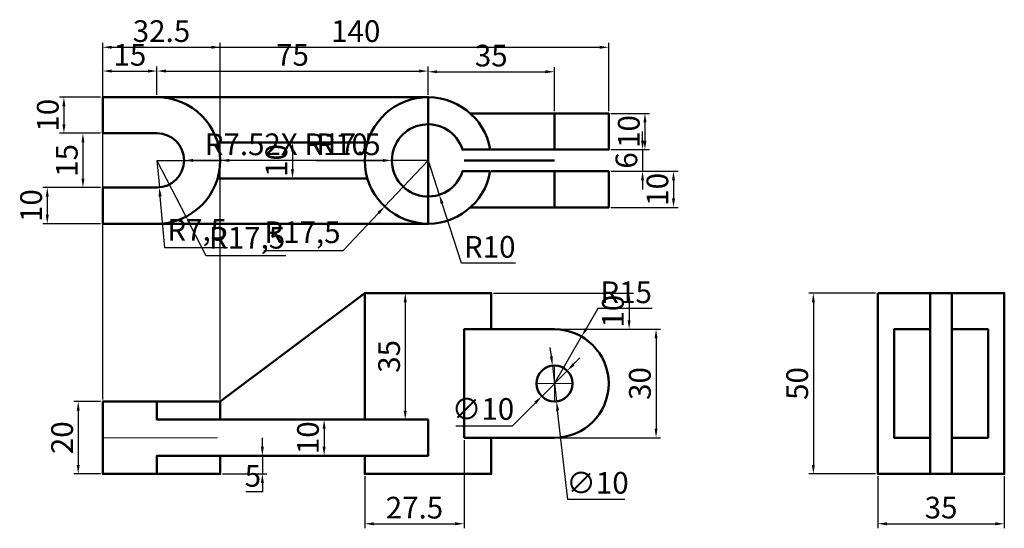
# Model space of a CAD drawing. Units: millimetres. Extents: x 147 to 419, y 95 to 236.
import ezdxf

# ---------------------------------------------------------------- set-up
doc = ezdxf.new("R2010")
doc.units = ezdxf.units.MM
doc.linetypes.add('CENTER', pattern=[50.8, 31.75, -6.35, 6.35, -6.35])
for name, color, linetype, lineweight in [('M-CNTR', 1, 'CENTER', 18), ('M-DIMS', 2, 'Continuous', 25), ('M-OUTL', 7, 'Continuous', 50)]:
    doc.layers.add(name, color=color, linetype=linetype, lineweight=lineweight)
doc.styles.get("Standard").update_dxf_attribs({"font": 'arial.ttf'})
doc.dimstyles.new('ISO-25', dxfattribs={"dimtxt": 6, "dimasz": 2.5, "dimexe": 1.25, "dimexo": 0.625, "dimtad": 1, "dimtoh": 1, "dimdec": 1, "dimtxsty": 'Standard', "dimcen": 2.5, "dimadec": 0, "dimazin": 0, "dimtfac": 1, "dimtdec": 1, "dimtmove": 0, "dimatfit": 3, "dimfxl": 1, "dimarcsym": 0})

# ---------------------------------------------------------------- blocks, each defined once
blk = doc.blocks.new('*D1')
at = {"layer": 'Defpoints', "color": 0, "transparency": 16777216}
for p in [(384.43, 159.98), (366.59, 109.98), (384.43, 109.98)]:
    blk.add_point(p, dxfattribs=at)
at = {"layer": 'M-DIMS', "color": 0, "lineweight": -2, "transparency": 16777216}
for p, q in [((383.8, 159.98), (365.34, 159.98)), ((366.59, 157.48), (366.59, 112.48)), ((383.8, 109.98), (365.34, 109.98))]:
    blk.add_line(p, q, dxfattribs=at)
at = {"layer": 'M-DIMS', "color": 0, "transparency": 16777216}
for points in [[(366.17, 157.48), (367.01, 157.48), (366.59, 159.98)], [(366.17, 112.48), (367.01, 112.48), (366.59, 109.98)]]:
    blk.add_solid(points, dxfattribs=at)
at = {"layer": 'M-DIMS', "color": 0, "transparency": 16777216, "insert": (362.9, 134.98), "char_height": 6, "attachment_point": 5, "rotation": 90}
blk.add_mtext('50', dxfattribs=at)
blk = doc.blocks.new('*D2')
at = {"layer": 'Defpoints', "color": 0, "transparency": 16777216}
for p in [(294.96, 149.98), (294.96, 119.98), (323.06, 119.98)]:
    blk.add_point(p, dxfattribs=at)
at = {"layer": 'M-DIMS', "color": 0, "lineweight": -2, "transparency": 16777216}
for p, q in [((295.58, 149.98), (324.31, 149.98)), ((323.06, 147.48), (323.06, 122.48)), ((295.58, 119.98), (324.31, 119.98))]:
    blk.add_line(p, q, dxfattribs=at)
at = {"layer": 'M-DIMS', "color": 0, "transparency": 16777216}
for points in [[(322.64, 147.48), (323.48, 147.48), (323.06, 149.98)], [(322.64, 122.48), (323.48, 122.48), (323.06, 119.98)]]:
    blk.add_solid(points, dxfattribs=at)
at = {"layer": 'M-DIMS', "color": 0, "transparency": 16777216, "insert": (319.37, 134.98), "char_height": 6, "attachment_point": 5, "rotation": 90}
blk.add_mtext('30', dxfattribs=at)
blk = doc.blocks.new('*D3')
at = {"layer": 'Defpoints', "color": 0, "transparency": 16777216}
for p in [(277.46, 159.98), (277.46, 149.98), (315.6, 149.98)]:
    blk.add_point(p, dxfattribs=at)
at = {"layer": 'M-DIMS', "color": 0, "lineweight": -2, "transparency": 16777216}
for p, q in [((278.08, 159.98), (316.85, 159.98)), ((315.6, 157.48), (315.6, 152.48)), ((278.08, 149.98), (316.85, 149.98))]:
    blk.add_line(p, q, dxfattribs=at)
at = {"layer": 'M-DIMS', "color": 0, "transparency": 16777216}
for points in [[(315.18, 157.48), (316.01, 157.48), (315.6, 159.98)], [(315.18, 152.48), (316.01, 152.48), (315.6, 149.98)]]:
    blk.add_solid(points, dxfattribs=at)
at = {"layer": 'M-DIMS', "color": 0, "transparency": 16777216, "insert": (311.91, 154.98), "char_height": 6, "attachment_point": 5, "rotation": 90}
blk.add_mtext('10', dxfattribs=at)
blk = doc.blocks.new('*D4')
at = {"layer": 'Defpoints', "color": 0, "transparency": 16777216}
for p in [(294.38, 139.94), (295.53, 130.01)]:
    blk.add_point(p, dxfattribs=at)
at = {"layer": 'M-DIMS', "color": 0, "lineweight": -2, "transparency": 16777216}
for p, q in [((294.09, 142.43), (293.8, 144.91)), ((294.38, 139.94), (295.53, 130.01)), ((298.68, 102.87), (295.82, 127.53)), ((314.41, 102.87), (298.68, 102.87))]:
    blk.add_line(p, q, dxfattribs=at)
at = {"layer": 'M-DIMS', "color": 0, "transparency": 16777216}
for points in [[(294.51, 142.47), (293.68, 142.38), (294.38, 139.94)], [(296.24, 127.57), (295.41, 127.48), (295.53, 130.01)]]:
    blk.add_solid(points, dxfattribs=at)
at = {"layer": 'M-DIMS', "color": 0, "transparency": 16777216, "insert": (306.86, 106.73), "char_height": 6, "attachment_point": 5}
blk.add_mtext('∅10', dxfattribs=at)
blk = doc.blocks.new('*D5')
at = {"layer": 'Defpoints', "color": 0, "transparency": 16777216}
for p in [(259.96, 159.98), (253.66, 124.98), (259.96, 124.98)]:
    blk.add_point(p, dxfattribs=at)
at = {"layer": 'M-DIMS', "color": 0, "lineweight": -2, "transparency": 16777216}
for p, q in [((259.33, 159.98), (252.41, 159.98)), ((253.66, 157.48), (253.66, 127.48)), ((259.33, 124.98), (252.41, 124.98))]:
    blk.add_line(p, q, dxfattribs=at)
at = {"layer": 'M-DIMS', "color": 0, "transparency": 16777216}
for points in [[(253.24, 157.48), (254.07, 157.48), (253.66, 159.98)], [(253.24, 127.48), (254.07, 127.48), (253.66, 124.98)]]:
    blk.add_solid(points, dxfattribs=at)
at = {"layer": 'M-DIMS', "color": 0, "transparency": 16777216, "insert": (249.97, 142.48), "char_height": 6, "attachment_point": 5, "rotation": 90}
blk.add_mtext('35', dxfattribs=at)
blk = doc.blocks.new('*D6')
at = {"layer": 'Defpoints', "color": 0, "transparency": 16777216}
for p in [(231.21, 124.98), (231.21, 114.98), (231.21, 114.98)]:
    blk.add_point(p, dxfattribs=at)
at = {"layer": 'M-DIMS', "color": 0, "lineweight": -2, "transparency": 16777216}
for p, q in [((231.83, 124.98), (232.46, 124.98)), ((231.21, 122.48), (231.21, 117.48)), ((231.83, 114.98), (232.46, 114.98))]:
    blk.add_line(p, q, dxfattribs=at)
at = {"layer": 'M-DIMS', "color": 0, "transparency": 16777216}
for points in [[(230.79, 122.48), (231.62, 122.48), (231.21, 124.98)], [(230.79, 117.48), (231.62, 117.48), (231.21, 114.98)]]:
    blk.add_solid(points, dxfattribs=at)
at = {"layer": 'M-DIMS', "color": 0, "transparency": 16777216, "insert": (227.52, 119.98), "char_height": 6, "attachment_point": 5, "rotation": 90}
blk.add_mtext('10', dxfattribs=at)
blk = doc.blocks.new('*D7')
at = {"layer": 'Defpoints', "color": 0, "transparency": 16777216}
for p in [(169.96, 129.98), (163.17, 109.98), (169.96, 109.98)]:
    blk.add_point(p, dxfattribs=at)
at = {"layer": 'M-DIMS', "color": 0, "lineweight": -2, "transparency": 16777216}
for p, q in [((169.33, 129.98), (161.92, 129.98)), ((163.17, 127.48), (163.17, 112.48)), ((169.33, 109.98), (161.92, 109.98))]:
    blk.add_line(p, q, dxfattribs=at)
at = {"layer": 'M-DIMS', "color": 0, "transparency": 16777216}
for points in [[(162.75, 127.48), (163.58, 127.48), (163.17, 129.98)], [(162.75, 112.48), (163.58, 112.48), (163.17, 109.98)]]:
    blk.add_solid(points, dxfattribs=at)
at = {"layer": 'M-DIMS', "color": 0, "transparency": 16777216, "insert": (159.48, 119.98), "char_height": 6, "attachment_point": 5, "rotation": 90}
blk.add_mtext('20', dxfattribs=at)
blk = doc.blocks.new('*D8')
at = {"layer": 'Defpoints', "color": 0, "transparency": 16777216}
for p in [(202.46, 114.98), (202.46, 109.98), (214.12, 109.98)]:
    blk.add_point(p, dxfattribs=at)
at = {"layer": 'M-DIMS', "color": 0, "lineweight": -2, "transparency": 16777216}
for p, q in [((214.12, 117.48), (214.12, 119.98)), ((203.08, 114.98), (215.37, 114.98)), ((214.12, 114.98), (214.12, 109.98)), ((203.08, 109.98), (215.37, 109.98)), ((214.12, 107.48), (214.12, 104.98)), ((214.12, 104.98), (209.52, 104.98))]:
    blk.add_line(p, q, dxfattribs=at)
at = {"layer": 'M-DIMS', "color": 0, "transparency": 16777216}
for points in [[(213.71, 117.48), (214.54, 117.48), (214.12, 114.98)], [(213.71, 107.48), (214.54, 107.48), (214.12, 109.98)]]:
    blk.add_solid(points, dxfattribs=at)
at = {"layer": 'M-DIMS', "color": 0, "transparency": 16777216, "insert": (211.51, 108.65), "char_height": 6, "attachment_point": 5}
blk.add_mtext('5', dxfattribs=at)
blk = doc.blocks.new('*D9')
at = {"layer": 'Defpoints', "color": 0, "transparency": 16777216}
for p in [(169.96, 214.19), (159.21, 204.19), (169.96, 204.19)]:
    blk.add_point(p, dxfattribs=at)
at = {"layer": 'M-DIMS', "color": 0, "lineweight": -2, "transparency": 16777216}
for p, q in [((169.33, 214.19), (157.96, 214.19)), ((159.21, 211.69), (159.21, 206.69)), ((169.33, 204.19), (157.96, 204.19))]:
    blk.add_line(p, q, dxfattribs=at)
at = {"layer": 'M-DIMS', "color": 0, "transparency": 16777216}
for points in [[(158.8, 211.69), (159.63, 211.69), (159.21, 214.19)], [(158.8, 206.69), (159.63, 206.69), (159.21, 204.19)]]:
    blk.add_solid(points, dxfattribs=at)
at = {"layer": 'M-DIMS', "color": 0, "transparency": 16777216, "insert": (155.52, 209.19), "char_height": 6, "attachment_point": 5, "rotation": 90}
blk.add_mtext('10', dxfattribs=at)
blk = doc.blocks.new('*D10')
at = {"layer": 'Defpoints', "color": 0, "transparency": 16777216}
for p in [(169.96, 204.19), (164.48, 189.19), (169.96, 189.19)]:
    blk.add_point(p, dxfattribs=at)
at = {"layer": 'M-DIMS', "color": 0, "lineweight": -2, "transparency": 16777216}
for p, q in [((169.33, 204.19), (163.23, 204.19)), ((164.48, 201.69), (164.48, 191.69)), ((169.33, 189.19), (163.23, 189.19))]:
    blk.add_line(p, q, dxfattribs=at)
at = {"layer": 'M-DIMS', "color": 0, "transparency": 16777216}
for points in [[(164.07, 201.69), (164.9, 201.69), (164.48, 204.19)], [(164.07, 191.69), (164.9, 191.69), (164.48, 189.19)]]:
    blk.add_solid(points, dxfattribs=at)
at = {"layer": 'M-DIMS', "color": 0, "transparency": 16777216, "insert": (160.79, 196.69), "char_height": 6, "attachment_point": 5, "rotation": 90}
blk.add_mtext('15', dxfattribs=at)
blk = doc.blocks.new('*D11')
at = {"layer": 'Defpoints', "color": 0, "transparency": 16777216}
for p in [(169.96, 189.19), (154.6, 179.19), (169.96, 179.19)]:
    blk.add_point(p, dxfattribs=at)
at = {"layer": 'M-DIMS', "color": 0, "lineweight": -2, "transparency": 16777216}
for p, q in [((169.33, 189.19), (153.35, 189.19)), ((154.6, 186.69), (154.6, 181.69)), ((169.33, 179.19), (153.35, 179.19))]:
    blk.add_line(p, q, dxfattribs=at)
at = {"layer": 'M-DIMS', "color": 0, "transparency": 16777216}
for points in [[(154.18, 186.69), (155.02, 186.69), (154.6, 189.19)], [(154.18, 181.69), (155.02, 181.69), (154.6, 179.19)]]:
    blk.add_solid(points, dxfattribs=at)
at = {"layer": 'M-DIMS', "color": 0, "transparency": 16777216, "insert": (150.91, 184.19), "char_height": 6, "attachment_point": 5, "rotation": 90}
blk.add_mtext('10', dxfattribs=at)
blk = doc.blocks.new('*D12')
at = {"layer": 'Defpoints', "color": 0, "transparency": 16777216}
for p in [(184.96, 221.42), (169.96, 214.19), (184.96, 214.19)]:
    blk.add_point(p, dxfattribs=at)
at = {"layer": 'M-DIMS', "color": 0, "lineweight": -2, "transparency": 16777216}
for p, q in [((169.96, 214.82), (169.96, 222.67)), ((172.46, 221.42), (182.46, 221.42)), ((184.96, 214.82), (184.96, 222.67))]:
    blk.add_line(p, q, dxfattribs=at)
at = {"layer": 'M-DIMS', "color": 0, "transparency": 16777216}
for points in [[(172.46, 221.84), (172.46, 221), (169.96, 221.42)], [(182.46, 221.84), (182.46, 221), (184.96, 221.42)]]:
    blk.add_solid(points, dxfattribs=at)
at = {"layer": 'M-DIMS', "color": 0, "transparency": 16777216, "insert": (177.46, 225.11), "char_height": 6, "attachment_point": 5}
blk.add_mtext('15', dxfattribs=at)
blk = doc.blocks.new('*D13')
at = {"layer": 'Defpoints', "color": 0, "transparency": 16777216}
for p in [(259.96, 221.42), (184.96, 218.74), (259.96, 214.19)]:
    blk.add_point(p, dxfattribs=at)
at = {"layer": 'M-DIMS', "color": 0, "lineweight": -2, "transparency": 16777216}
for p, q in [((184.96, 219.37), (184.96, 222.67)), ((187.46, 221.42), (257.46, 221.42)), ((259.96, 214.82), (259.96, 222.67))]:
    blk.add_line(p, q, dxfattribs=at)
at = {"layer": 'M-DIMS', "color": 0, "transparency": 16777216}
for points in [[(187.46, 221.84), (187.46, 221), (184.96, 221.42)], [(257.46, 221.84), (257.46, 221), (259.96, 221.42)]]:
    blk.add_solid(points, dxfattribs=at)
at = {"layer": 'M-DIMS', "color": 0, "transparency": 16777216, "insert": (222.46, 225.1), "char_height": 6, "attachment_point": 5}
blk.add_mtext('75', dxfattribs=at)
blk = doc.blocks.new('*D14')
at = {"layer": 'Defpoints', "color": 0, "transparency": 16777216}
for p in [(222.46, 201.69), (222.46, 191.69), (222.46, 191.69)]:
    blk.add_point(p, dxfattribs=at)
at = {"layer": 'M-DIMS', "color": 0, "lineweight": -2, "transparency": 16777216}
for p, q in [((223.08, 201.69), (223.71, 201.69)), ((222.46, 199.19), (222.46, 194.19)), ((223.08, 191.69), (223.71, 191.69))]:
    blk.add_line(p, q, dxfattribs=at)
at = {"layer": 'M-DIMS', "color": 0, "transparency": 16777216}
for points in [[(222.04, 199.19), (222.87, 199.19), (222.46, 201.69)], [(222.04, 194.19), (222.87, 194.19), (222.46, 191.69)]]:
    blk.add_solid(points, dxfattribs=at)
at = {"layer": 'M-DIMS', "color": 0, "transparency": 16777216, "insert": (218.77, 196.69), "char_height": 6, "attachment_point": 5, "rotation": 90}
blk.add_mtext('10', dxfattribs=at)
blk = doc.blocks.new('*D15')
at = {"layer": 'Defpoints', "color": 0, "transparency": 16777216}
for p in [(184.96, 196.69), (192.98, 181.14)]:
    blk.add_point(p, dxfattribs=at)
at = {"layer": 'M-DIMS', "color": 0, "lineweight": -2, "transparency": 16777216}
for p, q in [((184.96, 196.69), (192.98, 181.14)), ((198.58, 170.29), (194.13, 178.92)), ((220.58, 170.29), (198.58, 170.29))]:
    blk.add_line(p, q, dxfattribs=at)
at = {"layer": 'M-DIMS', "color": 0, "transparency": 16777216}
blk.add_solid([(194.5, 179.11), (193.76, 178.73), (192.98, 181.14)], dxfattribs=at)
at = {"layer": 'M-DIMS', "color": 0, "transparency": 16777216, "insert": (209.89, 174.52), "char_height": 6, "attachment_point": 5}
blk.add_mtext('R17,5', dxfattribs=at)
blk = doc.blocks.new('*D16')
at = {"layer": 'Defpoints', "color": 0, "transparency": 16777216}
for p in [(184.96, 196.69), (185.62, 189.22)]:
    blk.add_point(p, dxfattribs=at)
at = {"layer": 'M-DIMS', "color": 0, "lineweight": -2, "transparency": 16777216}
for p, q in [((184.96, 196.69), (185.62, 189.22)), ((187.11, 172.48), (185.84, 186.73)), ((204.44, 172.48), (187.11, 172.48))]:
    blk.add_line(p, q, dxfattribs=at)
at = {"layer": 'M-DIMS', "color": 0, "transparency": 16777216}
blk.add_solid([(186.26, 186.77), (185.43, 186.7), (185.62, 189.22)], dxfattribs=at)
at = {"layer": 'M-DIMS', "color": 0, "transparency": 16777216, "insert": (196.09, 176.7), "char_height": 6, "attachment_point": 5}
blk.add_mtext('R7,5', dxfattribs=at)
blk = doc.blocks.new('*D17')
at = {"layer": 'Defpoints', "color": 0, "transparency": 16777216}
for p in [(259.96, 196.69), (263.07, 187.19)]:
    blk.add_point(p, dxfattribs=at)
at = {"layer": 'M-DIMS', "color": 0, "lineweight": -2, "transparency": 16777216}
for p, q in [((259.96, 196.69), (263.07, 187.19)), ((269.25, 168.31), (263.85, 184.82)), ((284.19, 168.31), (269.25, 168.31))]:
    blk.add_line(p, q, dxfattribs=at)
at = {"layer": 'M-DIMS', "color": 0, "transparency": 16777216}
blk.add_solid([(264.24, 184.95), (263.45, 184.69), (263.07, 187.19)], dxfattribs=at)
at = {"layer": 'M-DIMS', "color": 0, "transparency": 16777216, "insert": (277.03, 172), "char_height": 6, "attachment_point": 5}
blk.add_mtext('R10', dxfattribs=at)
blk = doc.blocks.new('*D18')
at = {"layer": 'Defpoints', "color": 0, "transparency": 16777216}
for p in [(259.96, 196.69), (247.96, 183.96)]:
    blk.add_point(p, dxfattribs=at)
at = {"layer": 'M-DIMS', "color": 0, "lineweight": -2, "transparency": 16777216}
for p, q in [((259.96, 196.69), (247.96, 183.96)), ((236.52, 171.82), (246.24, 182.14)), ((214.53, 171.82), (236.52, 171.82))]:
    blk.add_line(p, q, dxfattribs=at)
at = {"layer": 'M-DIMS', "color": 0, "transparency": 16777216}
blk.add_solid([(245.94, 182.42), (246.55, 181.85), (247.96, 183.96)], dxfattribs=at)
at = {"layer": 'M-DIMS', "color": 0, "transparency": 16777216, "insert": (225.21, 176.05), "char_height": 6, "attachment_point": 5}
blk.add_mtext('R17,5', dxfattribs=at)
blk = doc.blocks.new('*D19')
at = {"layer": 'Defpoints', "color": 0, "transparency": 16777216}
for p in [(309.96, 209.69), (309.96, 199.69), (319.99, 199.69)]:
    blk.add_point(p, dxfattribs=at)
at = {"layer": 'M-DIMS', "color": 0, "lineweight": -2, "transparency": 16777216}
for p, q in [((310.58, 209.69), (321.24, 209.69)), ((319.99, 207.19), (319.99, 202.19)), ((310.58, 199.69), (321.24, 199.69))]:
    blk.add_line(p, q, dxfattribs=at)
at = {"layer": 'M-DIMS', "color": 0, "transparency": 16777216}
for points in [[(319.57, 207.19), (320.4, 207.19), (319.99, 209.69)], [(319.57, 202.19), (320.4, 202.19), (319.99, 199.69)]]:
    blk.add_solid(points, dxfattribs=at)
at = {"layer": 'M-DIMS', "color": 0, "transparency": 16777216, "insert": (316.3, 204.69), "char_height": 6, "attachment_point": 5, "rotation": 90}
blk.add_mtext('10', dxfattribs=at)
blk = doc.blocks.new('*D20')
at = {"layer": 'Defpoints', "color": 0, "transparency": 16777216}
for p in [(309.96, 199.69), (309.96, 193.69), (319.33, 193.69)]:
    blk.add_point(p, dxfattribs=at)
at = {"layer": 'M-DIMS', "color": 0, "lineweight": -2, "transparency": 16777216}
for p, q in [((319.33, 202.19), (319.33, 204.69)), ((310.58, 199.69), (320.58, 199.69)), ((319.33, 199.69), (319.33, 193.69)), ((310.58, 193.69), (320.58, 193.69)), ((319.33, 191.19), (319.33, 188.69))]:
    blk.add_line(p, q, dxfattribs=at)
at = {"layer": 'M-DIMS', "color": 0, "transparency": 16777216}
for points in [[(318.91, 202.19), (319.74, 202.19), (319.33, 199.69)], [(318.91, 191.19), (319.74, 191.19), (319.33, 193.69)]]:
    blk.add_solid(points, dxfattribs=at)
at = {"layer": 'M-DIMS', "color": 0, "transparency": 16777216, "insert": (315.64, 196.69), "char_height": 6, "attachment_point": 5, "rotation": 90}
blk.add_mtext('6', dxfattribs=at)
blk = doc.blocks.new('*D21')
at = {"layer": 'Defpoints', "color": 0, "transparency": 16777216}
for p in [(309.96, 193.69), (309.96, 183.69), (327.89, 183.69)]:
    blk.add_point(p, dxfattribs=at)
at = {"layer": 'M-DIMS', "color": 0, "lineweight": -2, "transparency": 16777216}
for p, q in [((310.58, 193.69), (329.14, 193.69)), ((327.89, 191.19), (327.89, 186.19)), ((310.58, 183.69), (329.14, 183.69))]:
    blk.add_line(p, q, dxfattribs=at)
at = {"layer": 'M-DIMS', "color": 0, "transparency": 16777216}
for points in [[(327.48, 191.19), (328.31, 191.19), (327.89, 193.69)], [(327.48, 186.19), (328.31, 186.19), (327.89, 183.69)]]:
    blk.add_solid(points, dxfattribs=at)
at = {"layer": 'M-DIMS', "color": 0, "transparency": 16777216, "insert": (324.21, 188.69), "char_height": 6, "attachment_point": 5, "rotation": 90}
blk.add_mtext('10', dxfattribs=at)
blk = doc.blocks.new('*D22')
at = {"layer": 'Defpoints', "color": 0, "transparency": 16777216}
for p in [(294.96, 221.22), (259.96, 214.19), (294.96, 209.69)]:
    blk.add_point(p, dxfattribs=at)
at = {"layer": 'M-DIMS', "color": 0, "lineweight": -2, "transparency": 16777216}
for p, q in [((259.96, 214.82), (259.96, 222.47)), ((262.46, 221.22), (292.46, 221.22)), ((294.96, 210.32), (294.96, 222.47))]:
    blk.add_line(p, q, dxfattribs=at)
at = {"layer": 'M-DIMS', "color": 0, "transparency": 16777216}
for points in [[(262.46, 221.64), (262.46, 220.81), (259.96, 221.22)], [(292.46, 221.64), (292.46, 220.81), (294.96, 221.22)]]:
    blk.add_solid(points, dxfattribs=at)
at = {"layer": 'M-DIMS', "color": 0, "transparency": 16777216, "insert": (277.46, 224.91), "char_height": 6, "attachment_point": 5}
blk.add_mtext('35', dxfattribs=at)
blk = doc.blocks.new('*D23')
at = {"layer": 'Defpoints', "color": 0, "transparency": 16777216}
for p in [(309.96, 227.99), (169.96, 214.19), (309.96, 209.69)]:
    blk.add_point(p, dxfattribs=at)
at = {"layer": 'M-DIMS', "color": 0, "lineweight": -2, "transparency": 16777216}
for p, q in [((169.96, 214.82), (169.96, 229.24)), ((309.96, 210.32), (309.96, 229.24)), ((172.46, 227.99), (307.46, 227.99))]:
    blk.add_line(p, q, dxfattribs=at)
at = {"layer": 'M-DIMS', "color": 0, "transparency": 16777216}
for points in [[(172.46, 228.41), (172.46, 227.58), (169.96, 227.99)], [(307.46, 228.41), (307.46, 227.58), (309.96, 227.99)]]:
    blk.add_solid(points, dxfattribs=at)
at = {"layer": 'M-DIMS', "color": 0, "transparency": 16777216, "insert": (239.96, 231.68), "char_height": 6, "attachment_point": 5}
blk.add_mtext('140', dxfattribs=at)
blk = doc.blocks.new('*D24')
at = {"layer": 'Defpoints', "color": 0, "transparency": 16777216}
for p in [(269.96, 119.98), (242.46, 109.98), (269.96, 96.18)]:
    blk.add_point(p, dxfattribs=at)
at = {"layer": 'M-DIMS', "color": 0, "lineweight": -2, "transparency": 16777216}
for p, q in [((269.96, 119.35), (269.96, 94.93)), ((242.46, 109.35), (242.46, 94.93)), ((244.96, 96.18), (267.46, 96.18))]:
    blk.add_line(p, q, dxfattribs=at)
at = {"layer": 'M-DIMS', "color": 0, "transparency": 16777216}
for points in [[(244.96, 96.59), (244.96, 95.76), (242.46, 96.18)], [(267.46, 96.59), (267.46, 95.76), (269.96, 96.18)]]:
    blk.add_solid(points, dxfattribs=at)
at = {"layer": 'M-DIMS', "color": 0, "transparency": 16777216, "insert": (256.21, 99.86), "char_height": 6, "attachment_point": 5}
blk.add_mtext('27.5', dxfattribs=at)
blk = doc.blocks.new('*D25')
at = {"layer": 'Defpoints', "color": 0, "transparency": 16777216}
for p in [(202.46, 227.99), (169.96, 129.98), (202.46, 129.98)]:
    blk.add_point(p, dxfattribs=at)
at = {"layer": 'M-DIMS', "color": 0, "lineweight": -2, "transparency": 16777216}
for p, q in [((169.96, 130.6), (169.96, 229.24)), ((202.46, 130.6), (202.46, 229.24)), ((172.46, 227.99), (199.96, 227.99))]:
    blk.add_line(p, q, dxfattribs=at)
at = {"layer": 'M-DIMS', "color": 0, "transparency": 16777216}
for points in [[(172.46, 228.41), (172.46, 227.58), (169.96, 227.99)], [(199.96, 228.41), (199.96, 227.58), (202.46, 227.99)]]:
    blk.add_solid(points, dxfattribs=at)
at = {"layer": 'M-DIMS', "color": 0, "transparency": 16777216, "insert": (186.21, 231.69), "char_height": 6, "attachment_point": 5}
blk.add_mtext('32.5', dxfattribs=at)
blk = doc.blocks.new('*D26')
at = {"layer": 'Defpoints', "color": 0, "transparency": 16777216}
for p in [(384.43, 109.98), (419.43, 109.98), (419.43, 96.18)]:
    blk.add_point(p, dxfattribs=at)
at = {"layer": 'M-DIMS', "color": 0, "lineweight": -2, "transparency": 16777216}
for p, q in [((384.43, 109.35), (384.43, 94.93)), ((419.43, 109.35), (419.43, 94.93)), ((386.93, 96.18), (416.93, 96.18))]:
    blk.add_line(p, q, dxfattribs=at)
at = {"layer": 'M-DIMS', "color": 0, "transparency": 16777216}
for points in [[(386.93, 96.59), (386.93, 95.76), (384.43, 96.18)], [(416.93, 96.59), (416.93, 95.76), (419.43, 96.18)]]:
    blk.add_solid(points, dxfattribs=at)
at = {"layer": 'M-DIMS', "color": 0, "transparency": 16777216, "insert": (401.93, 99.87), "char_height": 6, "attachment_point": 5}
blk.add_mtext('35', dxfattribs=at)
blk = doc.blocks.new('*D27')
at = {"layer": 'Defpoints', "color": 0, "transparency": 16777216}
for p in [(184.96, 196.69), (192.46, 196.69)]:
    blk.add_point(p, dxfattribs=at)
at = {"layer": 'M-DIMS', "color": 0, "lineweight": -2, "transparency": 16777216}
for p, q in [((184.96, 196.69), (192.46, 196.69)), ((197.46, 196.69), (194.96, 196.69)), ((214.79, 196.69), (197.46, 196.69))]:
    blk.add_line(p, q, dxfattribs=at)
at = {"layer": 'M-DIMS', "color": 0, "transparency": 16777216}
blk.add_solid([(194.96, 197.11), (194.96, 196.28), (192.46, 196.69)], dxfattribs=at)
at = {"layer": 'M-DIMS', "color": 0, "transparency": 16777216, "insert": (206.44, 200.37), "char_height": 6, "attachment_point": 5}
blk.add_mtext('R7.5', dxfattribs=at)
blk = doc.blocks.new('*D28')
at = {"layer": 'Defpoints', "color": 0, "transparency": 16777216}
for p in [(184.96, 196.69), (202.46, 196.69)]:
    blk.add_point(p, dxfattribs=at)
at = {"layer": 'M-DIMS', "color": 0, "lineweight": -2, "transparency": 16777216}
for p, q in [((184.96, 196.69), (202.46, 196.69)), ((212.96, 196.69), (204.96, 196.69)), ((247.95, 196.69), (212.96, 196.69))]:
    blk.add_line(p, q, dxfattribs=at)
at = {"layer": 'M-DIMS', "color": 0, "transparency": 16777216}
blk.add_solid([(204.96, 197.11), (204.96, 196.28), (202.46, 196.69)], dxfattribs=at)
at = {"layer": 'M-DIMS', "color": 0, "transparency": 16777216, "insert": (230.76, 200.38), "char_height": 6, "attachment_point": 5}
blk.add_mtext('2X R17.5', dxfattribs=at)
blk = doc.blocks.new('*D29')
at = {"layer": 'Defpoints', "color": 0, "transparency": 16777216}
for p in [(249.96, 196.69), (259.96, 196.69)]:
    blk.add_point(p, dxfattribs=at)
at = {"layer": 'M-DIMS', "color": 0, "lineweight": -2, "transparency": 16777216}
for p, q in [((229.01, 196.69), (243.96, 196.69)), ((243.96, 196.69), (247.46, 196.69)), ((259.96, 196.69), (249.96, 196.69))]:
    blk.add_line(p, q, dxfattribs=at)
at = {"layer": 'M-DIMS', "color": 0, "transparency": 16777216}
blk.add_solid([(247.46, 197.11), (247.46, 196.28), (249.96, 196.69)], dxfattribs=at)
at = {"layer": 'M-DIMS', "color": 0, "transparency": 16777216, "insert": (236.17, 200.38), "char_height": 6, "attachment_point": 5}
blk.add_mtext('R10', dxfattribs=at)
blk = doc.blocks.new('*D30')
at = {"layer": 'Defpoints', "color": 0, "transparency": 16777216}
for p in [(302.47, 147.96), (294.96, 134.98)]:
    blk.add_point(p, dxfattribs=at)
at = {"layer": 'M-DIMS', "color": 0, "lineweight": -2, "transparency": 16777216}
for p, q in [((306.99, 155.74), (303.73, 150.12)), ((321.99, 155.74), (306.99, 155.74)), ((294.96, 134.98), (302.47, 147.96))]:
    blk.add_line(p, q, dxfattribs=at)
at = {"layer": 'M-DIMS', "color": 0, "transparency": 16777216}
blk.add_solid([(303.37, 150.33), (304.09, 149.91), (302.47, 147.96)], dxfattribs=at)
at = {"layer": 'M-DIMS', "color": 0, "transparency": 16777216, "insert": (314.8, 159.43), "char_height": 6, "attachment_point": 5}
blk.add_mtext('R15', dxfattribs=at)
blk = doc.blocks.new('*D31')
at = {"layer": 'Defpoints', "color": 0, "transparency": 16777216}
for p in [(298.48, 138.52), (291.43, 131.43)]:
    blk.add_point(p, dxfattribs=at)
at = {"layer": 'M-DIMS', "color": 0, "lineweight": -2, "transparency": 16777216}
for p, q in [((300.25, 140.29), (302.01, 142.07)), ((298.48, 138.52), (291.43, 131.43)), ((283.35, 123.3), (289.67, 129.66)), ((267.62, 123.3), (283.35, 123.3))]:
    blk.add_line(p, q, dxfattribs=at)
at = {"layer": 'M-DIMS', "color": 0, "transparency": 16777216}
for points in [[(299.95, 140.59), (300.54, 140), (298.48, 138.52)], [(289.37, 129.95), (289.96, 129.36), (291.43, 131.43)]]:
    blk.add_solid(points, dxfattribs=at)
at = {"layer": 'M-DIMS', "color": 0, "transparency": 16777216, "insert": (275.17, 127.16), "char_height": 6, "attachment_point": 5}
blk.add_mtext('∅10', dxfattribs=at)

msp = doc.modelspace()

# ---------------------------------------------------------------- linework, layer by layer
at = {"layer": 'M-CNTR'}
for p, q in [((294.96, 139.98), (294.96, 129.98)), ((289.96, 134.98), (299.96, 134.98)), ((169.96, 119.98), (202.46, 119.98))]:
    msp.add_line(p, q, dxfattribs=at)
at = {"layer": 'M-OUTL'}
for p, q in [((169.96, 204.19), (169.96, 204.19)), ((201.73, 201.69), (243.19, 201.69)), ((202.46, 201.69), (242.46, 201.69)), ((277.46, 199.69), (294.96, 199.69)), ((277.46, 193.69), (294.96, 193.69)), ((201.73, 191.69), (243.19, 191.69)), ((242.46, 159.98), (242.46, 124.98)), ((398.93, 159.98), (398.93, 109.98)), ((404.93, 159.98), (404.93, 109.98))]:
    msp.add_line(p, q, dxfattribs=at)
for points in [[(169.96, 204.19), (169.96, 214.19), (259.96, 214.19), (259.96, 179.19), (169.96, 179.19), (169.96, 189.19), (184.96, 189.19, 1), (184.96, 204.19)], [(277.2, 193.69), (269.5, 193.69, -6.513131), (269.5, 199.69), (277.2, 199.69, 11.580313)], [(269.96, 119.98), (294.96, 119.98, 1), (294.96, 149.98), (269.96, 149.98)]]:
    msp.add_lwpolyline(points, format="xyb", close=True, dxfattribs=at)
for points in [[(271.67, 209.69), (294.96, 209.69), (309.96, 209.69), (309.96, 199.69), (294.96, 199.69), (294.96, 209.69)], [(269.96, 196.69), (277.46, 196.69), (294.96, 196.69)], [(271.67, 183.69), (294.96, 183.69), (309.96, 183.69), (309.96, 193.69), (294.96, 193.69), (294.96, 183.69)], [(202.46, 129.98), (202.46, 124.98), (259.96, 124.98), (259.96, 114.98), (202.46, 114.98), (202.46, 109.98), (169.96, 109.98), (169.96, 129.98), (202.46, 129.98), (242.46, 159.98), (277.46, 159.98), (277.46, 149.98)], [(398.93, 149.98), (388.93, 149.98), (388.93, 119.98), (398.93, 119.98)], [(404.93, 149.98), (414.93, 149.98), (414.93, 119.98), (404.93, 119.98)], [(184.96, 129.98), (184.96, 124.98), (202.46, 124.98)], [(242.46, 114.98), (242.46, 109.98), (277.46, 109.98), (277.46, 119.98)], [(202.46, 114.98), (184.96, 114.98), (184.96, 109.98)]]:
    msp.add_lwpolyline(points, dxfattribs=at)
msp.add_lwpolyline([(384.43, 159.98), (419.43, 159.98), (419.43, 109.98), (384.43, 109.98)], close=True, dxfattribs=at)
msp.add_circle((294.96, 134.98), 5, dxfattribs=at)
msp.add_arc((184.96, 196.69), 17.5, 270, 90, dxfattribs=at)

# ---------------------------------------------------------------- dimensions: what is measured, and where the dimension line sits
at = {"layer": 'M-DIMS'}
for base, p1, p2, override, picture, middle in [((309.96, 227.99), (169.96, 214.19), (309.96, 209.69), {"dimdec": 0, "dimlfac": 1, "dimrnd": 0, "dimzin": 0, "dimdsep": 46, "dimlunit": 2}, '*D23', (239.96, 231.68)), ((202.46, 227.99), (169.96, 129.98), (202.46, 129.98), {"dimdec": 1, "dimlfac": 1, "dimrnd": 0, "dimzin": 0, "dimdsep": 46, "dimlunit": 2}, '*D25', (186.21, 231.69)), ((184.96, 221.42), (169.96, 214.19), (184.96, 214.19), {"dimclrd": 0, "dimclre": 0, "dimclrt": 0}, '*D12', (177.46, 225.11)), ((259.96, 221.42), (184.96, 218.74), (259.96, 214.19), {"dimclrd": 0, "dimclre": 0, "dimclrt": 0}, '*D13', (222.46, 225.1)), ((294.96, 221.22), (259.96, 214.19), (294.96, 209.69), {"dimclrd": 0, "dimclre": 0, "dimclrt": 0}, '*D22', (277.46, 224.91)), ((269.96, 96.18), (242.46, 109.98), (269.96, 119.98), {"dimdec": 1, "dimlfac": 1, "dimrnd": 0, "dimzin": 0, "dimdsep": 46, "dimlunit": 2}, '*D24', (256.21, 99.86)), ((419.43, 96.18), (384.43, 109.98), (419.43, 109.98), {"dimdec": 0, "dimlfac": 1, "dimrnd": 0, "dimzin": 0, "dimdsep": 46, "dimlunit": 2}, '*D26', (401.93, 99.87))]:
    dim = msp.add_linear_dim(base=base, p1=p1, p2=p2, dimstyle='ISO-25', override=override, dxfattribs=at)
    dim.commit()
    dim.dimension.update_dxf_attribs({"geometry": picture, "text_midpoint": middle})
for base, p1, p2, picture, middle in [((159.21, 204.19), (169.96, 214.19), (169.96, 204.19), '*D9', (155.52, 209.19)), ((319.99, 199.69), (309.96, 209.69), (309.96, 199.69), '*D19', (316.3, 204.69)), ((319.33, 193.69), (309.96, 199.69), (309.96, 193.69), '*D20', (315.64, 196.69)), ((164.48, 189.19), (169.96, 204.19), (169.96, 189.19), '*D10', (160.79, 196.69)), ((222.46, 191.69), (222.46, 201.69), (222.46, 191.69), '*D14', (218.77, 196.69)), ((327.89, 183.69), (309.96, 193.69), (309.96, 183.69), '*D21', (324.21, 188.69)), ((154.6, 179.19), (169.96, 189.19), (169.96, 179.19), '*D11', (150.91, 184.19)), ((253.66, 124.98), (259.96, 159.98), (259.96, 124.98), '*D5', (249.97, 142.48)), ((315.6, 149.98), (277.46, 159.98), (277.46, 149.98), '*D3', (311.91, 154.98)), ((366.59, 109.98), (384.43, 159.98), (384.43, 109.98), '*D1', (362.9, 134.98)), ((323.06, 119.98), (294.96, 149.98), (294.96, 119.98), '*D2', (319.37, 134.98)), ((163.17, 109.98), (169.96, 129.98), (169.96, 109.98), '*D7', (159.48, 119.98)), ((231.21, 114.98), (231.21, 124.98), (231.21, 114.98), '*D6', (227.52, 119.98)), ((214.12, 109.98), (202.46, 114.98), (202.46, 109.98), '*D8', (211.51, 108.65))]:
    dim = msp.add_linear_dim(base=base, p1=p1, p2=p2, angle=90, dimstyle='ISO-25', override={"dimclrd": 0, "dimclre": 0, "dimclrt": 0}, dxfattribs=at)
    dim.commit()
    dim.dimension.update_dxf_attribs({"geometry": picture, "text_midpoint": middle})
dim = msp.add_radius_dim(center=(184.96, 196.69), mpoint=(202.46, 196.69), text='2X <>', dimstyle='ISO-25', override={"dimdec": 1, "dimlfac": 1, "dimrnd": 0, "dimzin": 0, "dimdsep": 46, "dimlunit": 2}, dxfattribs=at)
dim.commit()
dim.dimension.update_dxf_attribs({"geometry": '*D28', "text_midpoint": (212.96, 196.7), "dimtype": 164})
for mpoint, override, picture, middle in [((192.46, 196.69), {"dimdec": 1, "dimlfac": 1, "dimrnd": 0, "dimzin": 0, "dimdsep": 46, "dimlunit": 2}, '*D27', (206.44, 200.37)), ((192.98, 181.14), {"dimclrd": 0, "dimclre": 0, "dimclrt": 0}, '*D15', (209.89, 174.52))]:
    dim = msp.add_radius_dim(center=(184.96, 196.69), mpoint=mpoint, dimstyle='ISO-25', override=override, dxfattribs=at)
    dim.commit()
    dim.dimension.update_dxf_attribs({"geometry": picture, "text_midpoint": middle})
for center, mpoint, override, picture, middle in [((259.96, 196.69), (249.96, 196.69), {"dimdec": 0, "dimlfac": 1, "dimrnd": 0, "dimzin": 0, "dimdsep": 46, "dimlunit": 2}, '*D29', (243.96, 196.7)), ((184.96, 196.69), (185.62, 189.22), {"dimclrd": 0, "dimclre": 0, "dimclrt": 0}, '*D16', (196.09, 172.48)), ((259.96, 196.69), (247.96, 183.96), {"dimclrd": 0, "dimclre": 0, "dimclrt": 0}, '*D18', (225.21, 171.82)), ((259.96, 196.69), (263.07, 187.19), {"dimclrd": 0, "dimclre": 0, "dimclrt": 0}, '*D17', (277.03, 168.31)), ((294.96, 134.98), (302.47, 147.96), {"dimdec": 0, "dimlfac": 1, "dimrnd": 0, "dimzin": 0, "dimdsep": 46, "dimlunit": 2}, '*D30', (314.8, 155.74))]:
    dim = msp.add_radius_dim(center=center, mpoint=mpoint, dimstyle='ISO-25', override=override, dxfattribs=at)
    dim.commit()
    dim.dimension.update_dxf_attribs({"geometry": picture, "text_midpoint": middle, "dimtype": 164})
for p1, p2, override, picture, middle in [((294.38, 139.94), (295.53, 130.01), {"dimclrd": 0, "dimclre": 0, "dimclrt": 0}, '*D4', (306.86, 102.87)), ((298.48, 138.52), (291.43, 131.43), {"dimdec": 0, "dimlfac": 1, "dimrnd": 0, "dimzin": 0, "dimdsep": 46, "dimlunit": 2}, '*D31', (275.17, 123.3))]:
    dim = msp.add_diameter_dim_2p(p1=p1, p2=p2, dimstyle='ISO-25', override=override, dxfattribs=at)
    dim.commit()
    dim.dimension.update_dxf_attribs({"geometry": picture, "text_midpoint": middle, "dimtype": 163})

doc.saveas('drawing.dxf')
